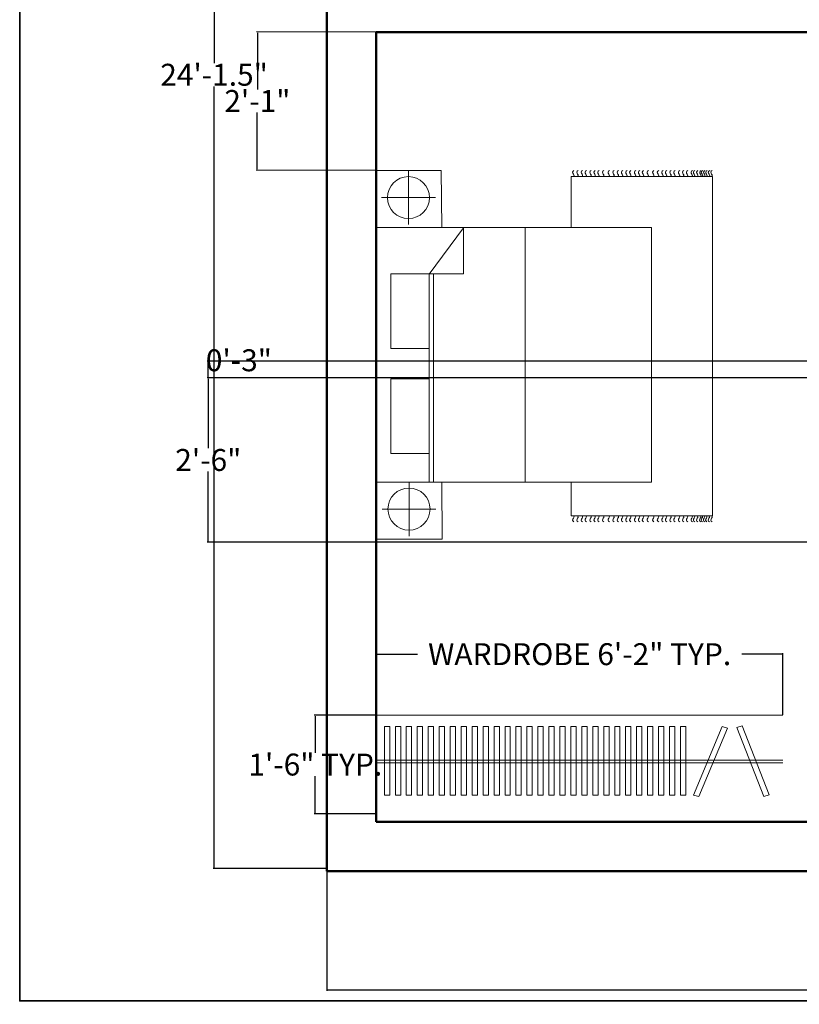
# Model space of a CAD drawing. Units: inches. Extents: x 124 to 591, y 365 to 713.
# Tile 1 of 5: x 124 to 266, y 365 to 545. Entities that reach past the tile are written whole.
import ezdxf

# ---------------------------------------------------------------- set-up
doc = ezdxf.new("R2010")
doc.units = ezdxf.units.IN
doc.header["$MEASUREMENT"] = 0
for name, color, linetype, lineweight in [('A-ANNO-DIMS', 2, 'Continuous', 18), ('A-ANNO-TTLB', 7, 'Continuous', 35), ('A-FLOR-CASE', 8, 'Continuous', 18), ('A-WALL', 7, 'Continuous', 50), ('furniture', 8, 'Continuous', 13)]:
    doc.layers.add(name, color=color, linetype=linetype, lineweight=lineweight)
doc.styles.get("Standard").update_dxf_attribs({"font": 'arial.ttf'})
doc.dimstyles.get("Standard").update_dxf_attribs({"dimtxt": 4, "dimasz": 0.18, "dimexe": 0.18, "dimexo": 0.0625, "dimgap": 0.09, "dimtad": 0, "dimtih": 1, "dimtoh": 1, "dimdec": 1, "dimzin": 0, "dimdsep": 46, "dimlunit": 3, "dimtxsty": 'Standard', "dimcen": 0.09, "dimclrd": 6, "dimclrt": 3, "dimadec": 0, "dimazin": 0, "dimtfac": 1, "dimtdec": 1, "dimtofl": 0, "dimtmove": 0, "dimatfit": 3, "dimfxl": 1, "dimtfillclr": 6, "dimtolj": 1, "dimtzin": 0, "dimarcsym": 0})

# ---------------------------------------------------------------- blocks, each defined once
blk = doc.blocks.new('CARPET')
at = {"layer": 'furniture'}
for p, q in [((-51.53, -98.11), (-51.53, -55.12)), ((-51.53, -55.12), (-41.27, -55.12)), ((36, -55.12), (51.55, -55.12)), ((51.55, -55.12), (51.55, -98.11)), ((51.55, -98.11), (-51.53, -98.11))]:
    blk.add_line(p, q, dxfattribs=at)
for points, knots in [([(-53.37, -55.99), (-53.22, -55.8), (-52.9, -55.41), (-52.34, -55.8), (-51.89, -56.08), (-51.65, -55.91), (-51.53, -55.83)], [0, 0, 0, 0, 0.653278, 1.290138, 1.740457, 2.114451, 2.114451, 2.114451, 2.114451]), ([(-53.37, -57.26), (-53.22, -57.07), (-52.9, -56.67), (-52.34, -57.07), (-51.89, -57.35), (-51.65, -57.17), (-51.53, -57.1)], [0, 0, 0, 0, 0.653278, 1.290138, 1.740457, 2.114451, 2.114451, 2.114451, 2.114451]), ([(53.37, -55.99), (53.22, -55.8), (52.9, -55.41), (52.34, -55.8), (51.89, -56.08), (51.65, -55.91), (51.53, -55.83)], [0, 0, 0, 0, 0.653278, 1.290138, 1.740457, 2.114451, 2.114451, 2.114451, 2.114451]), ([(53.37, -57.26), (53.22, -57.07), (52.9, -56.67), (52.34, -57.07), (51.89, -57.35), (51.65, -57.17), (51.53, -57.1)], [0, 0, 0, 0, 0.653278, 1.290138, 1.740457, 2.114451, 2.114451, 2.114451, 2.114451]), ([(-53.37, -58.59), (-53.22, -58.4), (-52.9, -58.01), (-52.34, -58.4), (-51.89, -58.68), (-51.65, -58.5), (-51.53, -58.43)], [0, 0, 0, 0, 0.653278, 1.290138, 1.740457, 2.114451, 2.114451, 2.114451, 2.114451]), ([(-53.37, -59.78), (-53.22, -59.58), (-52.9, -59.19), (-52.34, -59.58), (-51.89, -59.86), (-51.65, -59.69), (-51.53, -59.61)], [0, 0, 0, 0, 0.653278, 1.290138, 1.740457, 2.114451, 2.114451, 2.114451, 2.114451]), ([(53.37, -58.59), (53.22, -58.4), (52.9, -58.01), (52.34, -58.4), (51.89, -58.68), (51.65, -58.5), (51.53, -58.43)], [0, 0, 0, 0, 0.653278, 1.290138, 1.740457, 2.114451, 2.114451, 2.114451, 2.114451]), ([(53.37, -59.78), (53.22, -59.58), (52.9, -59.19), (52.34, -59.58), (51.89, -59.86), (51.65, -59.69), (51.53, -59.61)], [0, 0, 0, 0, 0.653278, 1.290138, 1.740457, 2.114451, 2.114451, 2.114451, 2.114451]), ([(-53.37, -61.22), (-53.22, -61.02), (-52.9, -60.63), (-52.34, -61.02), (-51.89, -61.3), (-51.65, -61.13), (-51.53, -61.05)], [0, 0, 0, 0, 0.653278, 1.290138, 1.740457, 2.114451, 2.114451, 2.114451, 2.114451]), ([(-53.37, -62.44), (-53.22, -62.25), (-52.9, -61.86), (-52.34, -62.25), (-51.89, -62.53), (-51.65, -62.36), (-51.53, -62.28)], [0, 0, 0, 0, 0.653278, 1.290138, 1.740457, 2.114451, 2.114451, 2.114451, 2.114451]), ([(53.37, -61.22), (53.22, -61.02), (52.9, -60.63), (52.34, -61.02), (51.89, -61.3), (51.65, -61.13), (51.53, -61.05)], [0, 0, 0, 0, 0.653278, 1.290138, 1.740457, 2.114451, 2.114451, 2.114451, 2.114451]), ([(53.37, -62.44), (53.22, -62.25), (52.9, -61.86), (52.34, -62.25), (51.89, -62.53), (51.65, -62.36), (51.53, -62.28)], [0, 0, 0, 0, 0.653278, 1.290138, 1.740457, 2.114451, 2.114451, 2.114451, 2.114451]), ([(-53.37, -63.63), (-53.22, -63.43), (-52.9, -63.04), (-52.34, -63.43), (-51.89, -63.72), (-51.65, -63.54), (-51.53, -63.46)], [0, 0, 0, 0, 0.653278, 1.290138, 1.740457, 2.114451, 2.114451, 2.114451, 2.114451]), ([(-53.37, -65.07), (-53.22, -64.87), (-52.9, -64.48), (-52.34, -64.87), (-51.89, -65.15), (-51.65, -64.98), (-51.53, -64.9)], [0, 0, 0, 0, 0.653278, 1.290138, 1.740457, 2.114451, 2.114451, 2.114451, 2.114451]), ([(53.37, -63.63), (53.22, -63.43), (52.9, -63.04), (52.34, -63.43), (51.89, -63.72), (51.65, -63.54), (51.53, -63.46)], [0, 0, 0, 0, 0.653278, 1.290138, 1.740457, 2.114451, 2.114451, 2.114451, 2.114451]), ([(53.37, -65.07), (53.22, -64.87), (52.9, -64.48), (52.34, -64.87), (51.89, -65.15), (51.65, -64.98), (51.53, -64.9)], [0, 0, 0, 0, 0.653278, 1.290138, 1.740457, 2.114451, 2.114451, 2.114451, 2.114451]), ([(-53.37, -66.76), (-53.22, -66.56), (-52.9, -66.17), (-52.34, -66.56), (-51.89, -66.84), (-51.65, -66.67), (-51.53, -66.59)], [0, 0, 0, 0, 0.653278, 1.290138, 1.740457, 2.114451, 2.114451, 2.114451, 2.114451]), ([(-53.37, -68.2), (-53.22, -68), (-52.9, -67.61), (-52.34, -68), (-51.89, -68.28), (-51.65, -68.11), (-51.53, -68.03)], [0, 0, 0, 0, 0.653278, 1.290138, 1.740457, 2.114451, 2.114451, 2.114451, 2.114451]), ([(53.37, -66.76), (53.22, -66.56), (52.9, -66.17), (52.34, -66.56), (51.89, -66.84), (51.65, -66.67), (51.53, -66.59)], [0, 0, 0, 0, 0.653278, 1.290138, 1.740457, 2.114451, 2.114451, 2.114451, 2.114451]), ([(53.37, -68.2), (53.22, -68), (52.9, -67.61), (52.34, -68), (51.89, -68.28), (51.65, -68.11), (51.53, -68.03)], [0, 0, 0, 0, 0.653278, 1.290138, 1.740457, 2.114451, 2.114451, 2.114451, 2.114451]), ([(-53.37, -69.53), (-53.22, -69.33), (-52.9, -68.94), (-52.34, -69.33), (-51.89, -69.61), (-51.65, -69.44), (-51.53, -69.36)], [0, 0, 0, 0, 0.653278, 1.290138, 1.740457, 2.114451, 2.114451, 2.114451, 2.114451]), ([(-53.37, -70.79), (-53.22, -70.6), (-52.9, -70.21), (-52.34, -70.6), (-51.89, -70.88), (-51.65, -70.7), (-51.53, -70.63)], [0, 0, 0, 0, 0.653278, 1.290138, 1.740457, 2.114451, 2.114451, 2.114451, 2.114451]), ([(-53.37, -72.12), (-53.22, -71.93), (-52.9, -71.54), (-52.34, -71.93), (-51.89, -72.21), (-51.65, -72.04), (-51.53, -71.96)], [0, 0, 0, 0, 0.653278, 1.290138, 1.740457, 2.114451, 2.114451, 2.114451, 2.114451]), ([(53.37, -69.53), (53.22, -69.33), (52.9, -68.94), (52.34, -69.33), (51.89, -69.61), (51.65, -69.44), (51.53, -69.36)], [0, 0, 0, 0, 0.653278, 1.290138, 1.740457, 2.114451, 2.114451, 2.114451, 2.114451]), ([(53.37, -70.79), (53.22, -70.6), (52.9, -70.21), (52.34, -70.6), (51.89, -70.88), (51.65, -70.7), (51.53, -70.63)], [0, 0, 0, 0, 0.653278, 1.290138, 1.740457, 2.114451, 2.114451, 2.114451, 2.114451]), ([(53.37, -72.12), (53.22, -71.93), (52.9, -71.54), (52.34, -71.93), (51.89, -72.21), (51.65, -72.04), (51.53, -71.96)], [0, 0, 0, 0, 0.653278, 1.290138, 1.740457, 2.114451, 2.114451, 2.114451, 2.114451]), ([(-53.37, -73.31), (-53.22, -73.11), (-52.9, -72.72), (-52.34, -73.11), (-51.89, -73.4), (-51.65, -73.22), (-51.53, -73.14)], [0, 0, 0, 0, 0.653278, 1.290138, 1.740457, 2.114451, 2.114451, 2.114451, 2.114451]), ([(-53.37, -74.75), (-53.22, -74.55), (-52.9, -74.16), (-52.34, -74.55), (-51.89, -74.83), (-51.65, -74.66), (-51.53, -74.58)], [0, 0, 0, 0, 0.653278, 1.290138, 1.740457, 2.114451, 2.114451, 2.114451, 2.114451]), ([(53.37, -73.31), (53.22, -73.11), (52.9, -72.72), (52.34, -73.11), (51.89, -73.4), (51.65, -73.22), (51.53, -73.14)], [0, 0, 0, 0, 0.653278, 1.290138, 1.740457, 2.114451, 2.114451, 2.114451, 2.114451]), ([(53.37, -74.75), (53.22, -74.55), (52.9, -74.16), (52.34, -74.55), (51.89, -74.83), (51.65, -74.66), (51.53, -74.58)], [0, 0, 0, 0, 0.653278, 1.290138, 1.740457, 2.114451, 2.114451, 2.114451, 2.114451]), ([(-53.37, -75.98), (-53.22, -75.78), (-52.9, -75.39), (-52.34, -75.78), (-51.89, -76.06), (-51.65, -75.89), (-51.53, -75.81)], [0, 0, 0, 0, 0.653278, 1.290138, 1.740457, 2.114451, 2.114451, 2.114451, 2.114451]), ([(-53.37, -77.16), (-53.22, -76.96), (-52.9, -76.57), (-52.34, -76.96), (-51.89, -77.25), (-51.65, -77.07), (-51.53, -76.99)], [0, 0, 0, 0, 0.653278, 1.290138, 1.740457, 2.114451, 2.114451, 2.114451, 2.114451]), ([(53.37, -75.98), (53.22, -75.78), (52.9, -75.39), (52.34, -75.78), (51.89, -76.06), (51.65, -75.89), (51.53, -75.81)], [0, 0, 0, 0, 0.653278, 1.290138, 1.740457, 2.114451, 2.114451, 2.114451, 2.114451]), ([(53.37, -77.16), (53.22, -76.96), (52.9, -76.57), (52.34, -76.96), (51.89, -77.25), (51.65, -77.07), (51.53, -76.99)], [0, 0, 0, 0, 0.653278, 1.290138, 1.740457, 2.114451, 2.114451, 2.114451, 2.114451]), ([(-53.37, -78.6), (-53.22, -78.4), (-52.9, -78.01), (-52.34, -78.4), (-51.89, -78.68), (-51.65, -78.51), (-51.53, -78.43)], [0, 0, 0, 0, 0.653278, 1.290138, 1.740457, 2.114451, 2.114451, 2.114451, 2.114451]), ([(-53.37, -80.29), (-53.22, -80.09), (-52.9, -79.7), (-52.34, -80.09), (-51.89, -80.37), (-51.65, -80.2), (-51.53, -80.12)], [0, 0, 0, 0, 0.653278, 1.290138, 1.740457, 2.114451, 2.114451, 2.114451, 2.114451]), ([(53.37, -78.6), (53.22, -78.4), (52.9, -78.01), (52.34, -78.4), (51.89, -78.68), (51.65, -78.51), (51.53, -78.43)], [0, 0, 0, 0, 0.653278, 1.290138, 1.740457, 2.114451, 2.114451, 2.114451, 2.114451]), ([(53.37, -80.29), (53.22, -80.09), (52.9, -79.7), (52.34, -80.09), (51.89, -80.37), (51.65, -80.2), (51.53, -80.12)], [0, 0, 0, 0, 0.653278, 1.290138, 1.740457, 2.114451, 2.114451, 2.114451, 2.114451]), ([(-53.37, -81.73), (-53.22, -81.53), (-52.9, -81.14), (-52.34, -81.53), (-51.89, -81.81), (-51.65, -81.64), (-51.53, -81.56)], [0, 0, 0, 0, 0.653278, 1.290138, 1.740457, 2.114451, 2.114451, 2.114451, 2.114451]), ([(-53.37, -83.06), (-53.22, -82.86), (-52.9, -82.47), (-52.34, -82.86), (-51.89, -83.14), (-51.65, -82.97), (-51.53, -82.89)], [0, 0, 0, 0, 0.653278, 1.290138, 1.740457, 2.114451, 2.114451, 2.114451, 2.114451]), ([(-53.37, -84.18), (-53.22, -83.99), (-52.9, -83.6), (-52.34, -83.99), (-51.89, -84.27), (-51.65, -84.09), (-51.53, -84.02)], [0, 0, 0, 0, 0.653278, 1.290138, 1.740457, 2.114451, 2.114451, 2.114451, 2.114451]), ([(53.37, -81.73), (53.22, -81.53), (52.9, -81.14), (52.34, -81.53), (51.89, -81.81), (51.65, -81.64), (51.53, -81.56)], [0, 0, 0, 0, 0.653278, 1.290138, 1.740457, 2.114451, 2.114451, 2.114451, 2.114451]), ([(53.37, -83.06), (53.22, -82.86), (52.9, -82.47), (52.34, -82.86), (51.89, -83.14), (51.65, -82.97), (51.53, -82.89)], [0, 0, 0, 0, 0.653278, 1.290138, 1.740457, 2.114451, 2.114451, 2.114451, 2.114451]), ([(53.37, -84.18), (53.22, -83.99), (52.9, -83.6), (52.34, -83.99), (51.89, -84.27), (51.65, -84.09), (51.53, -84.02)], [0, 0, 0, 0, 0.653278, 1.290138, 1.740457, 2.114451, 2.114451, 2.114451, 2.114451]), ([(-53.37, -85.51), (-53.22, -85.32), (-52.9, -84.93), (-52.34, -85.32), (-51.89, -85.6), (-51.65, -85.42), (-51.53, -85.35)], [0, 0, 0, 0, 0.653278, 1.290138, 1.740457, 2.114451, 2.114451, 2.114451, 2.114451]), ([(-53.37, -86.7), (-53.22, -86.5), (-52.9, -86.11), (-52.34, -86.5), (-51.89, -86.78), (-51.65, -86.61), (-51.53, -86.53)], [0, 0, 0, 0, 0.653278, 1.290138, 1.740457, 2.114451, 2.114451, 2.114451, 2.114451]), ([(53.37, -85.51), (53.22, -85.32), (52.9, -84.93), (52.34, -85.32), (51.89, -85.6), (51.65, -85.42), (51.53, -85.35)], [0, 0, 0, 0, 0.653278, 1.290138, 1.740457, 2.114451, 2.114451, 2.114451, 2.114451]), ([(53.37, -86.7), (53.22, -86.5), (52.9, -86.11), (52.34, -86.5), (51.89, -86.78), (51.65, -86.61), (51.53, -86.53)], [0, 0, 0, 0, 0.653278, 1.290138, 1.740457, 2.114451, 2.114451, 2.114451, 2.114451]), ([(-53.37, -88.14), (-53.22, -87.94), (-52.9, -87.55), (-52.34, -87.94), (-51.89, -88.22), (-51.65, -88.05), (-51.53, -87.97)], [0, 0, 0, 0, 0.653278, 1.290138, 1.740457, 2.114451, 2.114451, 2.114451, 2.114451]), ([(-53.37, -89.36), (-53.22, -89.17), (-52.9, -88.78), (-52.34, -89.17), (-51.89, -89.45), (-51.65, -89.28), (-51.53, -89.2)], [0, 0, 0, 0, 0.653278, 1.290138, 1.740457, 2.114451, 2.114451, 2.114451, 2.114451]), ([(53.37, -88.14), (53.22, -87.94), (52.9, -87.55), (52.34, -87.94), (51.89, -88.22), (51.65, -88.05), (51.53, -87.97)], [0, 0, 0, 0, 0.653278, 1.290138, 1.740457, 2.114451, 2.114451, 2.114451, 2.114451]), ([(53.37, -89.36), (53.22, -89.17), (52.9, -88.78), (52.34, -89.17), (51.89, -89.45), (51.65, -89.28), (51.53, -89.2)], [0, 0, 0, 0, 0.653278, 1.290138, 1.740457, 2.114451, 2.114451, 2.114451, 2.114451]), ([(-53.37, -90.55), (-53.22, -90.35), (-52.9, -89.96), (-52.34, -90.35), (-51.89, -90.64), (-51.65, -90.46), (-51.53, -90.38)], [0, 0, 0, 0, 0.653278, 1.290138, 1.740457, 2.114451, 2.114451, 2.114451, 2.114451]), ([(-53.37, -91.99), (-53.22, -91.79), (-52.9, -91.4), (-52.34, -91.79), (-51.89, -92.07), (-51.65, -91.9), (-51.53, -91.82)], [0, 0, 0, 0, 0.653278, 1.290138, 1.740457, 2.114451, 2.114451, 2.114451, 2.114451]), ([(-53.37, -92.69), (-53.22, -92.48), (-52.9, -92.08), (-52.35, -92.49), (-51.89, -92.77), (-51.65, -92.6), (-51.53, -92.52)], [0, 0, 0, 0, 0.663904, 1.307406, 1.757725, 2.131719, 2.131719, 2.131719, 2.131719]), ([(53.37, -90.55), (53.22, -90.35), (52.9, -89.96), (52.34, -90.35), (51.9, -90.63), (51.66, -90.47), (51.55, -90.4)], [0, 0, 0, 0, 0.653278, 1.290138, 1.740457, 2.0926, 2.0926, 2.0926, 2.0926]), ([(53.37, -91.99), (53.22, -91.79), (52.9, -91.4), (52.34, -91.79), (51.9, -92.07), (51.66, -91.91), (51.55, -91.83)], [0, 0, 0, 0, 0.653278, 1.290138, 1.740457, 2.0926, 2.0926, 2.0926, 2.0926]), ([(53.37, -92.69), (53.22, -92.49), (52.9, -92.09), (52.34, -92.49), (51.9, -92.77), (51.66, -92.61), (51.55, -92.53)], [0, 0, 0, 0, 0.656792, 1.295826, 1.746145, 2.098292, 2.098292, 2.098292, 2.098292]), ([(-53.37, -93.61), (-53.22, -93.42), (-52.9, -93.03), (-52.34, -93.42), (-51.89, -93.7), (-51.65, -93.52), (-51.53, -93.45)], [0, 0, 0, 0, 0.653278, 1.290138, 1.740457, 2.114451, 2.114451, 2.114451, 2.114451]), ([(-53.37, -94.55), (-53.22, -94.35), (-52.9, -93.96), (-52.34, -94.35), (-51.89, -94.63), (-51.65, -94.46), (-51.53, -94.38)], [0, 0, 0, 0, 0.653278, 1.290138, 1.740457, 2.114451, 2.114451, 2.114451, 2.114451]), ([(-53.37, -95.05), (-53.22, -94.85), (-52.9, -94.46), (-52.34, -94.85), (-51.89, -95.14), (-51.65, -94.96), (-51.53, -94.88)], [0, 0, 0, 0, 0.653278, 1.290138, 1.740457, 2.114451, 2.114451, 2.114451, 2.114451]), ([(-53.37, -95.73), (-53.22, -95.54), (-52.9, -95.15), (-52.34, -95.54), (-51.89, -95.82), (-51.65, -95.65), (-51.53, -95.57)], [0, 0, 0, 0, 0.653278, 1.290138, 1.740457, 2.114451, 2.114451, 2.114451, 2.114451]), ([(53.37, -95.78), (53.22, -95.58), (52.9, -95.19), (52.34, -95.58), (51.89, -95.86), (51.65, -95.69), (51.53, -95.61)], [0, 0, 0, 0, 0.653278, 1.290138, 1.740457, 2.114451, 2.114451, 2.114451, 2.114451]), ([(53.37, -93.66), (53.22, -93.46), (52.9, -93.07), (52.34, -93.46), (51.9, -93.74), (51.66, -93.58), (51.55, -93.5)], [0, 0, 0, 0, 0.653278, 1.290138, 1.740457, 2.0926, 2.0926, 2.0926, 2.0926]), ([(53.37, -94.59), (53.22, -94.4), (52.9, -94.01), (52.34, -94.4), (51.9, -94.68), (51.66, -94.51), (51.55, -94.44)], [0, 0, 0, 0, 0.653278, 1.290138, 1.740457, 2.0926, 2.0926, 2.0926, 2.0926]), ([(53.37, -95.1), (53.22, -94.9), (52.9, -94.51), (52.34, -94.9), (51.9, -95.18), (51.66, -95.02), (51.55, -94.94)], [0, 0, 0, 0, 0.653278, 1.290138, 1.740457, 2.0926, 2.0926, 2.0926, 2.0926]), ([(-53.37, -96.38), (-53.22, -96.18), (-52.9, -95.79), (-52.34, -96.18), (-51.89, -96.47), (-51.65, -96.29), (-51.53, -96.21)], [0, 0, 0, 0, 0.653278, 1.290138, 1.740457, 2.114451, 2.114451, 2.114451, 2.114451]), ([(-53.37, -97.17), (-53.22, -96.98), (-52.9, -96.59), (-52.34, -96.98), (-51.89, -97.26), (-51.65, -97.08), (-51.53, -97.01)], [0, 0, 0, 0, 0.653278, 1.290138, 1.740457, 2.114451, 2.114451, 2.114451, 2.114451]), ([(-53.37, -97.99), (-53.22, -97.79), (-52.9, -97.4), (-52.34, -97.79), (-51.89, -98.08), (-51.65, -97.9), (-51.53, -97.82)], [0, 0, 0, 0, 0.653278, 1.290138, 1.740457, 2.114451, 2.114451, 2.114451, 2.114451]), ([(53.37, -96.43), (53.22, -96.23), (52.9, -95.84), (52.34, -96.23), (51.89, -96.51), (51.65, -96.34), (51.53, -96.26)], [0, 0, 0, 0, 0.653278, 1.290138, 1.740457, 2.114451, 2.114451, 2.114451, 2.114451]), ([(53.37, -97.22), (53.22, -97.02), (52.9, -96.63), (52.34, -97.02), (51.89, -97.3), (51.65, -97.13), (51.53, -97.05)], [0, 0, 0, 0, 0.653278, 1.290138, 1.740457, 2.114451, 2.114451, 2.114451, 2.114451]), ([(53.37, -97.99), (53.22, -97.79), (52.9, -97.4), (52.34, -97.79), (51.89, -98.08), (51.65, -97.9), (51.53, -97.82)], [0, 0, 0, 0, 0.653278, 1.290138, 1.740457, 2.114451, 2.114451, 2.114451, 2.114451])]:
    blk.add_open_spline(points, degree=3, knots=knots, dxfattribs=at)
blk = doc.blocks.new('A$C58D270C6')
at = {"layer": 'furniture'}
for p, q in [((9.09, 124.13), (9.09, 108.87)), ((1.46, 116.5), (16.73, 116.5)), ((14.97, 94.84), (24.62, 107.92)), ((24.62, 94.93), (24.62, 107.92)), ((42.08, 108), (42.08, 36)), ((14.97, 94.93), (24.62, 94.93)), ((14.97, 94.84), (14.97, 36)), ((16.22, 94.93), (16.22, 36)), ((9.25, 36), (9.25, 20.74)), ((1.62, 28.37), (16.88, 28.37))]:
    blk.add_line(p, q, dxfattribs=at)
for points in [[(18.5, 108), (18.34, 124.13), (-0.16, 124.13), (0, 108)], [(0, 108), (77.91, 108), (77.91, 36), (0, 36)], [(4.09, 94.93), (14.97, 94.93), (14.97, 73.83), (4.09, 73.83)], [(4.09, 65.23), (14.97, 65.23), (14.97, 44.13), (4.09, 44.13)], [(18.65, 19.87), (18.5, 36), (0, 36), (0.16, 19.87)]]:
    blk.add_lwpolyline(points, close=True, dxfattribs=at)
for centre in [(9.09, 116.5), (9.25, 28.37)]:
    blk.add_circle(centre, 5.95, dxfattribs=at)
at = {"layer": 'furniture', "xscale": 0.9312884925094044, "yscale": 0.9312884925094044, "zscale": 0.9312884925094044, "rotation": 90}
blk.add_blockref('CARPET', (3.79, 74.47), dxfattribs=at)
blk = doc.blocks.new('*D20')
at = {"layer": 'A-ANNO-DIMS', "color": 0, "lineweight": -2, "transparency": 16777216}
for p, q in [((180.08, 679.59), (159.36, 679.59)), ((159.54, 679.41), (159.54, 536.98)), ((159.54, 390.27), (159.54, 532.71)), ((180.08, 390.09), (159.36, 390.09))]:
    blk.add_line(p, q, dxfattribs=at)
at = {"layer": 'A-ANNO-DIMS', "color": 0, "transparency": 16777216}
for points in [[(159.51, 679.41), (159.57, 679.41), (159.54, 679.59)], [(159.51, 390.27), (159.57, 390.27), (159.54, 390.09)]]:
    blk.add_solid(points, dxfattribs=at)
at = {"layer": 'Defpoints', "color": 0, "transparency": 16777216}
for p in [(159.54, 679.59), (180.14, 679.59), (180.14, 390.09)]:
    blk.add_point(p, dxfattribs=at)
at = {"layer": 'A-ANNO-DIMS', "color": 0, "transparency": 16777216, "insert": (159.54, 534.84), "char_height": 4, "attachment_point": 5}
blk.add_mtext('\\A1;24\'-1.5"', dxfattribs=at)
blk = doc.blocks.new('WARDROBE-HANGING-RAIL')
for p, q in [((0, 18), (74.16, 18)), ((0, 0), (0, 18)), ((0, 9.79), (74.16, 9.79)), ((0, 9.29), (74.16, 9.29))]:
    blk.add_line(p, q)
for points in [[(1.47, 3.44), (1.47, 15.95), (2.44, 15.95), (2.44, 3.44)], [(3.47, 3.44), (3.47, 15.95), (4.44, 15.95), (4.44, 3.44)], [(5.47, 3.44), (5.47, 15.95), (6.44, 15.95), (6.44, 3.44)], [(7.47, 3.44), (7.47, 15.95), (8.44, 15.95), (8.44, 3.44)], [(7.47, 3.44), (7.47, 15.95), (8.44, 15.95), (8.44, 3.44)], [(9.47, 3.44), (9.47, 15.95), (10.44, 15.95), (10.44, 3.44)], [(11.47, 3.44), (11.47, 15.95), (12.44, 15.95), (12.44, 3.44)], [(13.47, 3.44), (13.47, 15.95), (14.44, 15.95), (14.44, 3.44)], [(15.47, 3.44), (15.47, 15.95), (16.44, 15.95), (16.44, 3.44)], [(17.47, 3.44), (17.47, 15.95), (18.44, 15.95), (18.44, 3.44)], [(19.47, 3.44), (19.47, 15.95), (20.44, 15.95), (20.44, 3.44)], [(19.47, 3.44), (19.47, 15.95), (20.44, 15.95), (20.44, 3.44)], [(21.47, 3.44), (21.47, 15.95), (22.44, 15.95), (22.44, 3.44)], [(23.47, 3.44), (23.47, 15.95), (24.44, 15.95), (24.44, 3.44)], [(25.47, 3.44), (25.47, 15.95), (26.44, 15.95), (26.44, 3.44)], [(27.47, 3.44), (27.47, 15.95), (28.44, 15.95), (28.44, 3.44)], [(29.47, 3.44), (29.47, 15.95), (30.44, 15.95), (30.44, 3.44)], [(31.47, 3.44), (31.47, 15.95), (32.44, 15.95), (32.44, 3.44)], [(31.47, 3.44), (31.47, 15.95), (32.44, 15.95), (32.44, 3.44)], [(33.47, 3.44), (33.47, 15.95), (34.44, 15.95), (34.44, 3.44)], [(35.47, 3.44), (35.47, 15.95), (36.44, 15.95), (36.44, 3.44)], [(37.47, 3.44), (37.47, 15.95), (38.44, 15.95), (38.44, 3.44)], [(39.47, 3.44), (39.47, 15.95), (40.44, 15.95), (40.44, 3.44)], [(41.47, 3.44), (41.47, 15.95), (42.44, 15.95), (42.44, 3.44)], [(43.47, 3.44), (43.47, 15.95), (44.44, 15.95), (44.44, 3.44)], [(43.47, 3.44), (43.47, 15.95), (44.44, 15.95), (44.44, 3.44)], [(45.47, 3.44), (45.47, 15.95), (46.44, 15.95), (46.44, 3.44)], [(47.47, 3.44), (47.47, 15.95), (48.44, 15.95), (48.44, 3.44)], [(49.47, 3.44), (49.47, 15.95), (50.44, 15.95), (50.44, 3.44)], [(51.47, 3.44), (51.47, 15.95), (52.44, 15.95), (52.44, 3.44)], [(53.47, 3.44), (53.47, 15.95), (54.44, 15.95), (54.44, 3.44)], [(55.47, 3.44), (55.47, 15.95), (56.44, 15.95), (56.44, 3.44)], [(57.87, 3.44), (58.83, 3.15), (64.04, 15.66), (63.08, 15.95)], [(70.7, 3.17), (71.66, 3.45), (66.73, 16.04), (65.77, 15.76)]]:
    blk.add_lwpolyline(points, close=True)
blk = doc.blocks.new('*D30')
at = {"layer": 'A-ANNO-DIMS', "color": 0, "lineweight": -2, "transparency": 16777216}
for p, q in [((189.14, 418.1), (189.14, 429.35)), ((263.3, 418.1), (263.3, 429.35))]:
    blk.add_line(p, q, dxfattribs=at)
at = {"layer": 'A-ANNO-DIMS', "color": 6, "lineweight": -2, "transparency": 16777216}
for p, q in [((189.32, 429.17), (196.62, 429.17)), ((263.12, 429.17), (255.81, 429.17))]:
    blk.add_line(p, q, dxfattribs=at)
at = {"layer": 'A-ANNO-DIMS', "color": 6, "transparency": 16777216}
for points in [[(189.32, 429.2), (189.32, 429.14), (189.14, 429.17)], [(263.12, 429.2), (263.12, 429.14), (263.3, 429.17)]]:
    blk.add_solid(points, dxfattribs=at)
at = {"layer": 'Defpoints', "color": 0, "transparency": 16777216}
for p in [(263.3, 429.17), (189.14, 418.04), (263.3, 418.04)]:
    blk.add_point(p, dxfattribs=at)
at = {"layer": 'A-ANNO-DIMS', "color": 3, "transparency": 16777216, "insert": (226.22, 429.17), "char_height": 4, "attachment_point": 5}
blk.add_mtext('\\A1;WARDROBE 6\'-2" TYP.', dxfattribs=at)
blk = doc.blocks.new('*D31')
at = {"layer": 'A-ANNO-DIMS', "color": 0, "lineweight": -2, "transparency": 16777216}
for p, q in [((189.08, 418.04), (177.83, 418.04)), ((189.08, 400.04), (177.83, 400.04))]:
    blk.add_line(p, q, dxfattribs=at)
at = {"layer": 'A-ANNO-DIMS', "color": 6, "lineweight": -2, "transparency": 16777216}
for p, q in [((178.01, 417.86), (178.01, 411.17)), ((178.01, 400.22), (178.01, 406.91))]:
    blk.add_line(p, q, dxfattribs=at)
at = {"layer": 'A-ANNO-DIMS', "color": 6, "transparency": 16777216}
for points in [[(177.98, 417.86), (178.04, 417.86), (178.01, 418.04)], [(177.98, 400.22), (178.04, 400.22), (178.01, 400.04)]]:
    blk.add_solid(points, dxfattribs=at)
at = {"layer": 'Defpoints', "color": 0, "transparency": 16777216}
for p in [(178.01, 418.04), (189.14, 418.04), (189.14, 400.04)]:
    blk.add_point(p, dxfattribs=at)
at = {"layer": 'A-ANNO-DIMS', "color": 3, "transparency": 16777216, "insert": (178.01, 409.04), "char_height": 4, "attachment_point": 5}
blk.add_mtext('\\A1;1\'-6" TYP.', dxfattribs=at)
blk = doc.blocks.new('*D44')
at = {"layer": 'A-ANNO-DIMS', "color": 0, "lineweight": -2, "transparency": 16777216}
for p, q in [((180.14, 389.53), (180.14, 367.76)), ((562.14, 389.53), (562.14, 367.76))]:
    blk.add_line(p, q, dxfattribs=at)
at = {"layer": 'A-ANNO-DIMS', "color": 6, "lineweight": -2, "transparency": 16777216}
for p, q in [((180.32, 367.94), (362.63, 367.94)), ((561.96, 367.94), (379.65, 367.94))]:
    blk.add_line(p, q, dxfattribs=at)
at = {"layer": 'A-ANNO-DIMS', "color": 6, "transparency": 16777216}
for points in [[(180.32, 367.97), (180.32, 367.91), (180.14, 367.94)], [(561.96, 367.97), (561.96, 367.91), (562.14, 367.94)]]:
    blk.add_solid(points, dxfattribs=at)
at = {"layer": 'Defpoints', "color": 0, "transparency": 16777216}
for p in [(180.14, 389.59), (562.14, 389.59), (562.14, 367.94)]:
    blk.add_point(p, dxfattribs=at)
at = {"layer": 'A-ANNO-DIMS', "color": 3, "transparency": 16777216, "insert": (371.14, 367.94), "char_height": 4, "attachment_point": 5}
blk.add_mtext('\\A1;31\'-10"', dxfattribs=at)
blk = doc.blocks.new('*D55')
at = {"layer": 'A-ANNO-DIMS', "color": 0, "lineweight": -2, "transparency": 16777216}
for p, q in [((325.58, 479.59), (158.31, 479.59)), ((325.58, 449.59), (158.31, 449.59))]:
    blk.add_line(p, q, dxfattribs=at)
at = {"layer": 'A-ANNO-DIMS', "color": 6, "lineweight": -2, "transparency": 16777216}
for p, q in [((158.49, 479.41), (158.49, 466.72)), ((158.49, 449.77), (158.49, 462.46))]:
    blk.add_line(p, q, dxfattribs=at)
at = {"layer": 'A-ANNO-DIMS', "color": 6, "transparency": 16777216}
for points in [[(158.46, 479.41), (158.52, 479.41), (158.49, 479.59)], [(158.46, 449.77), (158.52, 449.77), (158.49, 449.59)]]:
    blk.add_solid(points, dxfattribs=at)
at = {"layer": 'Defpoints', "color": 0, "transparency": 16777216}
for p in [(158.49, 479.59), (325.64, 479.59), (325.64, 449.59)]:
    blk.add_point(p, dxfattribs=at)
at = {"layer": 'A-ANNO-DIMS', "color": 3, "transparency": 16777216, "insert": (158.49, 464.59), "char_height": 4, "attachment_point": 5}
blk.add_mtext('\\A1;2\'-6"', dxfattribs=at)
blk = doc.blocks.new('*D56')
at = {"layer": 'A-ANNO-DIMS', "color": 0, "lineweight": -2, "transparency": 16777216}
for p, q in [((330.08, 482.59), (158.31, 482.59)), ((330.08, 479.59), (158.31, 479.59))]:
    blk.add_line(p, q, dxfattribs=at)
at = {"layer": 'A-ANNO-DIMS', "color": 6, "lineweight": -2, "transparency": 16777216}
for p, q in [((158.49, 482.59), (158.49, 482.77)), ((158.49, 482.77), (158.67, 482.77)), ((158.49, 479.77), (158.49, 482.41))]:
    blk.add_line(p, q, dxfattribs=at)
at = {"layer": 'A-ANNO-DIMS', "color": 6, "transparency": 16777216}
for points in [[(158.46, 482.41), (158.52, 482.41), (158.49, 482.59)], [(158.46, 479.77), (158.52, 479.77), (158.49, 479.59)]]:
    blk.add_solid(points, dxfattribs=at)
at = {"layer": 'Defpoints', "color": 0, "transparency": 16777216}
for p in [(158.49, 482.59), (330.14, 482.59), (330.14, 479.59)]:
    blk.add_point(p, dxfattribs=at)
at = {"layer": 'A-ANNO-DIMS', "color": 3, "transparency": 16777216, "insert": (164.07, 482.77), "char_height": 4, "attachment_point": 5}
blk.add_mtext('\\A1;0\'-3"', dxfattribs=at)
blk = doc.blocks.new('*D66')
at = {"layer": 'A-ANNO-DIMS', "color": 0, "lineweight": -2, "transparency": 16777216}
for p, q in [((189.08, 542.59), (167.31, 542.68)), ((188.98, 517.36), (167.21, 517.44))]:
    blk.add_line(p, q, dxfattribs=at)
at = {"layer": 'A-ANNO-DIMS', "color": 6, "lineweight": -2, "transparency": 16777216}
for p, q in [((167.49, 542.5), (167.45, 532.16)), ((167.39, 517.62), (167.43, 527.96))]:
    blk.add_line(p, q, dxfattribs=at)
at = {"layer": 'A-ANNO-DIMS', "color": 6, "transparency": 16777216}
for points in [[(167.46, 542.5), (167.52, 542.5), (167.49, 542.68)], [(167.36, 517.62), (167.42, 517.62), (167.39, 517.44)]]:
    blk.add_solid(points, dxfattribs=at)
at = {"layer": 'Defpoints', "color": 0, "transparency": 16777216}
for p in [(167.49, 542.68), (189.14, 542.59), (189.04, 517.36)]:
    blk.add_point(p, dxfattribs=at)
at = {"layer": 'A-ANNO-DIMS', "color": 3, "transparency": 16777216, "insert": (167.44, 530.06), "char_height": 4, "attachment_point": 5}
blk.add_mtext('\\A1;2\'-1"', dxfattribs=at)

msp = doc.modelspace()

# ---------------------------------------------------------------- linework, layer by layer
at = {"layer": 'A-ANNO-TTLB'}
msp.add_lwpolyline([(124.09, 712.7), (590.57, 712.7), (590.57, 365.95), (124.09, 365.95)], close=True, dxfattribs=at)
msp.add_lwpolyline([(124.09, 712.7), (590.57, 712.7), (590.57, 365.95), (124.09, 365.95)], close=True, dxfattribs=at)
at = {"layer": 'A-WALL'}
for p, q in [((180.14, 679.09), (180.14, 389.59)), ((189.14, 542.59), (339.14, 542.59)), ((189.14, 542.59), (189.14, 398.59)), ((189.14, 398.59), (325.64, 398.59)), ((180.14, 389.59), (562.14, 389.59))]:
    msp.add_line(p, q, dxfattribs=at)

# ---------------------------------------------------------------- block references
at = {"layer": 'A-FLOR-CASE'}
msp.add_blockref('WARDROBE-HANGING-RAIL', (189.14, 400.04), dxfattribs=at)
at = {"layer": 'furniture', "xscale": 0.6445294581626225, "yscale": 0.6445294581626225, "zscale": 0.6445294581626225}
msp.add_blockref('A$C58D270C6', (189.14, 437.35), dxfattribs=at)

# ---------------------------------------------------------------- dimensions: what is measured, and where the dimension line sits
at = {"layer": 'A-ANNO-DIMS'}
for base, p1, p2, angle, override, picture, middle in [((159.54, 679.59), (180.14, 390.09), (180.14, 679.59), 90, {"dimclrd": 0, "dimclre": 0, "dimclrt": 0}, '*D20', (159.54, 534.84)), ((167.49, 542.68), (189.04, 517.36), (189.14, 542.59), 89.7724, {"dimdec": 1, "dimlfac": 1, "dimrnd": 0, "dimzin": 1, "dimdsep": 46, "dimlunit": 4, "dimfrac": 2}, '*D66', (167.44, 530.06)), ((158.49, 482.59), (330.14, 479.59), (330.14, 482.59), 90, {"dimdec": 1, "dimlfac": 1, "dimrnd": 0, "dimzin": 1, "dimdsep": 46, "dimlunit": 4, "dimfrac": 2}, '*D56', (164.07, 482.77)), ((158.49, 479.59), (325.64, 449.59), (325.64, 479.59), 90, {"dimdec": 1, "dimlfac": 1, "dimrnd": 0, "dimzin": 1, "dimdsep": 46, "dimlunit": 4, "dimfrac": 2}, '*D55', (158.49, 464.59))]:
    dim = msp.add_linear_dim(base=base, p1=p1, p2=p2, angle=angle, dimstyle='Standard', override=override, dxfattribs=at)
    dim.commit()
    dim.dimension.update_dxf_attribs({"geometry": picture, "text_midpoint": middle})
dim = msp.add_linear_dim(base=(263.3, 429.17), p1=(189.14, 418.04), p2=(263.3, 418.04), text='WARDROBE <> TYP.', dimstyle='Standard', override={"dimdec": 1, "dimlfac": 1, "dimrnd": 0, "dimzin": 1, "dimdsep": 46, "dimlunit": 4, "dimfrac": 2}, dxfattribs=at)
dim.commit()
dim.dimension.update_dxf_attribs({"geometry": '*D30', "text_midpoint": (226.22, 429.17)})
dim = msp.add_linear_dim(base=(178.01, 418.04), p1=(189.14, 400.04), p2=(189.14, 418.04), angle=90, text='<> TYP.', dimstyle='Standard', override={"dimdec": 1, "dimlfac": 1, "dimrnd": 0, "dimzin": 1, "dimdsep": 46, "dimlunit": 4, "dimfrac": 2}, dxfattribs=at)
dim.commit()
dim.dimension.update_dxf_attribs({"geometry": '*D31', "text_midpoint": (178.01, 409.04)})
dim = msp.add_linear_dim(base=(562.14, 367.94), p1=(180.14, 389.59), p2=(562.14, 389.59), dimstyle='Standard', override={"dimdec": 1, "dimlfac": 1, "dimrnd": 0, "dimzin": 1, "dimdsep": 46, "dimlunit": 4, "dimfrac": 2}, dxfattribs=at)
dim.commit()
dim.dimension.update_dxf_attribs({"geometry": '*D44', "text_midpoint": (371.14, 367.94)})

doc.saveas('drawing.dxf')
